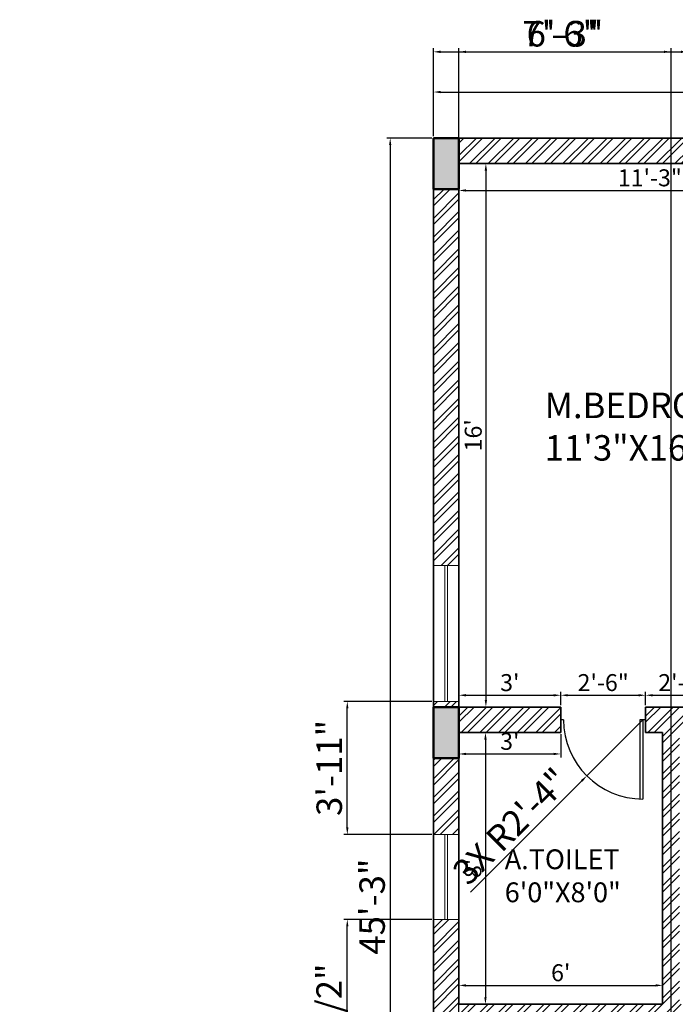
# Model space of a CAD drawing. Units: inches. Extents: x 4153 to 5577, y 785 to 1503.
# Tile 8 of 11: x 4865 to 5097, y 1138 to 1486. Entities that reach past the tile are written whole.
import ezdxf

# ---------------------------------------------------------------- set-up
doc = ezdxf.new("R2010")
doc.units = ezdxf.units.IN
for name, color, linetype, lineweight in [('A-ANNO-DIMS', 2, 'Continuous', 18), ('A-AREA-IDEN', 7, 'Continuous', 25), ('A-COLS', 7, 'Continuous', 50), ('A-DOOR', 3, 'Continuous', 25), ('A-GLAZ', 4, 'Continuous', 18), ('A-WALL', 7, 'Continuous', 35)]:
    doc.layers.add(name, color=color, linetype=linetype, lineweight=lineweight)
doc.layers.add('A-WALL-PATT', color=251, linetype='Continuous', lineweight=13, true_color=0x636466)
doc.styles.get("Standard").update_dxf_attribs({"font": 'arial.ttf'})
doc.dimstyles.new('ISO-25', dxfattribs={"dimtxt": 9, "dimasz": 2.5, "dimexe": 1.25, "dimexo": 0.625, "dimtad": 1, "dimlunit": 3, "dimtxsty": 'Standard', "dimcen": 2.5, "dimadec": 0, "dimazin": 0, "dimtfac": 1, "dimtmove": 0, "dimatfit": 3, "dimfxl": 1, "dimarcsym": 0})

# ---------------------------------------------------------------- blocks, each defined once
blk = doc.blocks.new('D2')
for p, q in [((1, 0), (1, 28)), ((2, 0), (2, 27.98)), ((0, 0), (2, 0)), ((29, 0), (30, 0))]:
    blk.add_line(p, q)
at = {"ltscale": 0.5}
blk.add_arc((1, 0), 28, 0, 90, dxfattribs=at)
blk = doc.blocks.new('*D23')
at = {"layer": 'A-ANNO-DIMS', "color": 0, "lineweight": -2, "transparency": 16777216}
for p, q in [((5011.25, 1445.11), (5011.25, 1461.99)), ((5518.25, 1445.11), (5518.25, 1461.99)), ((5013.75, 1460.74), (5515.75, 1460.74))]:
    blk.add_line(p, q, dxfattribs=at)
at = {"layer": 'A-ANNO-DIMS', "color": 0, "transparency": 16777216}
for points in [[(5013.75, 1461.16), (5013.75, 1460.33), (5011.25, 1460.74)], [(5515.75, 1461.16), (5515.75, 1460.33), (5518.25, 1460.74)]]:
    blk.add_solid(points, dxfattribs=at)
at = {"layer": 'Defpoints', "color": 0, "transparency": 16777216}
for p in [(5518.25, 1460.74), (5011.25, 1444.49), (5518.25, 1444.49)]:
    blk.add_point(p, dxfattribs=at)
at = {"layer": 'A-ANNO-DIMS', "color": 0, "transparency": 16777216, "insert": (5264.75, 1465.97), "char_height": 9, "attachment_point": 5}
blk.add_mtext('42\'-3"', dxfattribs=at)
blk = doc.blocks.new('*D24')
at = {"layer": 'A-ANNO-DIMS', "color": 0, "lineweight": -2, "transparency": 16777216}
for p, q in [((5010.63, 1444.49), (4994.72, 1444.49)), ((4995.97, 1441.99), (4995.97, 903.99)), ((5010.63, 901.49), (4994.72, 901.49))]:
    blk.add_line(p, q, dxfattribs=at)
at = {"layer": 'A-ANNO-DIMS', "color": 0, "transparency": 16777216}
for points in [[(4995.55, 1441.99), (4996.38, 1441.99), (4995.97, 1444.49)], [(4995.55, 903.99), (4996.38, 903.99), (4995.97, 901.49)]]:
    blk.add_solid(points, dxfattribs=at)
at = {"layer": 'Defpoints', "color": 0, "transparency": 16777216}
for p in [(5011.25, 1444.49), (4995.97, 901.49), (5011.25, 901.49)]:
    blk.add_point(p, dxfattribs=at)
at = {"layer": 'A-ANNO-DIMS', "color": 0, "transparency": 16777216, "insert": (4990.74, 1172.99), "char_height": 9, "attachment_point": 5, "rotation": 90}
blk.add_mtext('45\'-3"', dxfattribs=at)
blk = doc.blocks.new('*D25')
at = {"layer": 'A-ANNO-DIMS', "color": 0, "lineweight": -2, "transparency": 16777216}
for p, q in [((5020.25, 1434.86), (5020.25, 1424.72)), ((5155.25, 1434.86), (5155.25, 1424.72)), ((5022.75, 1425.97), (5152.75, 1425.97))]:
    blk.add_line(p, q, dxfattribs=at)
at = {"layer": 'A-ANNO-DIMS', "color": 0, "transparency": 16777216}
for points in [[(5022.75, 1426.39), (5022.75, 1425.56), (5020.25, 1425.97)], [(5152.75, 1426.39), (5152.75, 1425.56), (5155.25, 1425.97)]]:
    blk.add_solid(points, dxfattribs=at)
at = {"layer": 'Defpoints', "color": 0, "transparency": 16777216}
for p in [(5020.25, 1435.49), (5155.25, 1435.49), (5155.25, 1425.97)]:
    blk.add_point(p, dxfattribs=at)
at = {"layer": 'A-ANNO-DIMS', "color": 0, "transparency": 16777216, "insert": (5087.75, 1429.66), "char_height": 6, "attachment_point": 5}
blk.add_mtext('11\'-3"', dxfattribs=at)
blk = doc.blocks.new('*D26')
at = {"layer": 'A-ANNO-DIMS', "color": 0, "lineweight": -2, "transparency": 16777216}
for p, q in [((5020.88, 1435.49), (5031.04, 1435.49)), ((5029.79, 1432.99), (5029.79, 1245.99)), ((5020.88, 1243.49), (5031.04, 1243.49))]:
    blk.add_line(p, q, dxfattribs=at)
at = {"layer": 'A-ANNO-DIMS', "color": 0, "transparency": 16777216}
for points in [[(5029.37, 1432.99), (5030.21, 1432.99), (5029.79, 1435.49)], [(5029.37, 1245.99), (5030.21, 1245.99), (5029.79, 1243.49)]]:
    blk.add_solid(points, dxfattribs=at)
at = {"layer": 'Defpoints', "color": 0, "transparency": 16777216}
for p in [(5020.25, 1435.49), (5020.25, 1243.49), (5029.79, 1243.49)]:
    blk.add_point(p, dxfattribs=at)
at = {"layer": 'A-ANNO-DIMS', "color": 0, "transparency": 16777216, "insert": (5026.1, 1339.49), "char_height": 6, "attachment_point": 5, "rotation": 90}
blk.add_mtext("16'", dxfattribs=at)
blk = doc.blocks.new('*D27')
at = {"layer": 'A-ANNO-DIMS', "color": 0, "lineweight": -2, "transparency": 16777216}
for p, q in [((5020.25, 1244.11), (5020.25, 1248.91)), ((5056.25, 1244.11), (5056.25, 1248.91)), ((5022.75, 1247.66), (5053.75, 1247.66))]:
    blk.add_line(p, q, dxfattribs=at)
at = {"layer": 'A-ANNO-DIMS', "color": 0, "transparency": 16777216}
for points in [[(5022.75, 1248.07), (5022.75, 1247.24), (5020.25, 1247.66)], [(5053.75, 1248.07), (5053.75, 1247.24), (5056.25, 1247.66)]]:
    blk.add_solid(points, dxfattribs=at)
at = {"layer": 'Defpoints', "color": 0, "transparency": 16777216}
for p in [(5056.25, 1247.66), (5020.25, 1243.49), (5056.25, 1243.49)]:
    blk.add_point(p, dxfattribs=at)
at = {"layer": 'A-ANNO-DIMS', "color": 0, "transparency": 16777216, "insert": (5038.25, 1251.35), "char_height": 6, "attachment_point": 5}
blk.add_mtext("3'", dxfattribs=at)
blk = doc.blocks.new('*D28')
at = {"layer": 'A-ANNO-DIMS', "color": 0, "lineweight": -2, "transparency": 16777216}
for p, q in [((5056.25, 1244.11), (5056.25, 1248.91)), ((5086.25, 1244.11), (5086.25, 1248.91)), ((5058.75, 1247.66), (5083.75, 1247.66))]:
    blk.add_line(p, q, dxfattribs=at)
at = {"layer": 'A-ANNO-DIMS', "color": 0, "transparency": 16777216}
for points in [[(5058.75, 1248.07), (5058.75, 1247.24), (5056.25, 1247.66)], [(5083.75, 1248.07), (5083.75, 1247.24), (5086.25, 1247.66)]]:
    blk.add_solid(points, dxfattribs=at)
at = {"layer": 'Defpoints', "color": 0, "transparency": 16777216}
for p in [(5086.25, 1247.66), (5056.25, 1243.49), (5086.25, 1243.49)]:
    blk.add_point(p, dxfattribs=at)
at = {"layer": 'A-ANNO-DIMS', "color": 0, "transparency": 16777216, "insert": (5071.25, 1251.35), "char_height": 6, "attachment_point": 5}
blk.add_mtext('2\'-6"', dxfattribs=at)
blk = doc.blocks.new('*D29')
at = {"layer": 'A-ANNO-DIMS', "color": 0, "lineweight": -2, "transparency": 16777216}
for p, q in [((5086.25, 1244.11), (5086.25, 1248.91)), ((5113.25, 1244.11), (5113.25, 1248.91)), ((5088.75, 1247.66), (5110.75, 1247.66))]:
    blk.add_line(p, q, dxfattribs=at)
at = {"layer": 'A-ANNO-DIMS', "color": 0, "transparency": 16777216}
for points in [[(5088.75, 1248.07), (5088.75, 1247.24), (5086.25, 1247.66)], [(5110.75, 1248.07), (5110.75, 1247.24), (5113.25, 1247.66)]]:
    blk.add_solid(points, dxfattribs=at)
at = {"layer": 'Defpoints', "color": 0, "transparency": 16777216}
for p in [(5113.25, 1247.66), (5086.25, 1243.49), (5113.25, 1243.49)]:
    blk.add_point(p, dxfattribs=at)
at = {"layer": 'A-ANNO-DIMS', "color": 0, "transparency": 16777216, "insert": (5099.75, 1251.35), "char_height": 6, "attachment_point": 5}
blk.add_mtext('2\'-3"', dxfattribs=at)
blk = doc.blocks.new('*D41')
at = {"layer": 'A-ANNO-DIMS', "color": 0, "lineweight": -2, "transparency": 16777216}
for p, q in [((5020.25, 1233.86), (5020.25, 1225.67)), ((5056.25, 1233.86), (5056.25, 1225.67)), ((5022.75, 1226.92), (5053.75, 1226.92))]:
    blk.add_line(p, q, dxfattribs=at)
at = {"layer": 'A-ANNO-DIMS', "color": 0, "transparency": 16777216}
for points in [[(5022.75, 1227.34), (5022.75, 1226.51), (5020.25, 1226.92)], [(5053.75, 1227.34), (5053.75, 1226.51), (5056.25, 1226.92)]]:
    blk.add_solid(points, dxfattribs=at)
at = {"layer": 'Defpoints', "color": 0, "transparency": 16777216}
for p in [(5020.25, 1234.49), (5056.25, 1234.49), (5056.25, 1226.92)]:
    blk.add_point(p, dxfattribs=at)
at = {"layer": 'A-ANNO-DIMS', "color": 0, "transparency": 16777216, "insert": (5038.25, 1230.61), "char_height": 6, "attachment_point": 5}
blk.add_mtext("3'", dxfattribs=at)
blk = doc.blocks.new('*D42')
at = {"layer": 'A-ANNO-DIMS', "color": 0, "lineweight": -2, "transparency": 16777216}
for p, q in [((5020.88, 1234.49), (5030.89, 1234.49)), ((5029.64, 1231.99), (5029.64, 1140.99)), ((5020.88, 1138.49), (5030.89, 1138.49))]:
    blk.add_line(p, q, dxfattribs=at)
at = {"layer": 'A-ANNO-DIMS', "color": 0, "transparency": 16777216}
for points in [[(5029.22, 1231.99), (5030.06, 1231.99), (5029.64, 1234.49)], [(5029.22, 1140.99), (5030.06, 1140.99), (5029.64, 1138.49)]]:
    blk.add_solid(points, dxfattribs=at)
at = {"layer": 'Defpoints', "color": 0, "transparency": 16777216}
for p in [(5020.25, 1234.49), (5020.25, 1138.49), (5029.64, 1138.49)]:
    blk.add_point(p, dxfattribs=at)
at = {"layer": 'A-ANNO-DIMS', "color": 0, "transparency": 16777216, "insert": (5025.95, 1186.49), "char_height": 6, "attachment_point": 5, "rotation": 90}
blk.add_mtext("8'", dxfattribs=at)
blk = doc.blocks.new('*D43')
at = {"layer": 'A-ANNO-DIMS', "color": 0, "lineweight": -2, "transparency": 16777216}
for p, q in [((5020.25, 1139.11), (5020.25, 1146.42)), ((5022.75, 1145.17), (5089.75, 1145.17)), ((5092.25, 1139.11), (5092.25, 1146.42))]:
    blk.add_line(p, q, dxfattribs=at)
at = {"layer": 'A-ANNO-DIMS', "color": 0, "transparency": 16777216}
for points in [[(5022.75, 1145.59), (5022.75, 1144.75), (5020.25, 1145.17)], [(5089.75, 1145.59), (5089.75, 1144.75), (5092.25, 1145.17)]]:
    blk.add_solid(points, dxfattribs=at)
at = {"layer": 'Defpoints', "color": 0, "transparency": 16777216}
for p in [(5092.25, 1145.17), (5020.25, 1138.49), (5092.25, 1138.49)]:
    blk.add_point(p, dxfattribs=at)
at = {"layer": 'A-ANNO-DIMS', "color": 0, "transparency": 16777216, "insert": (5056.25, 1148.86), "char_height": 6, "attachment_point": 5}
blk.add_mtext("6'", dxfattribs=at)
blk = doc.blocks.new('WINDOW-48IN')
for p, q in [((0, 9), (0, 0)), ((48, 9), (48, 0)), ((0, 5), (48, 5)), ((0, 4), (48, 4))]:
    blk.add_line(p, q)
blk = doc.blocks.new('VENT-WINDOW-30IN')
for p, q in [((9, 30), (0, 30)), ((4, 0), (4, 30)), ((5, 0), (5, 30)), ((9, 0), (0, 0))]:
    blk.add_line(p, q)
blk = doc.blocks.new('COL-9X18IN')
at = {"transparency": 33554687}
h = blk.add_hatch(color=256, dxfattribs=at)
h.dxf.hatch_style = 1
h.paths.add_polyline_path([(9, 18), (0, 18), (0, 0), (9, 0)])
blk.add_lwpolyline([(0, 18), (9, 18), (9, 0), (0, 0)], close=True)
blk = doc.blocks.new('*D146')
at = {"layer": 'A-ANNO-DIMS', "color": 0, "lineweight": -2, "transparency": 16777216}
for p, q in [((5011.25, 1445.11), (5011.25, 1476.19)), ((5013.75, 1474.94), (5098.75, 1474.94)), ((5101.25, 1445.11), (5101.25, 1476.19))]:
    blk.add_line(p, q, dxfattribs=at)
at = {"layer": 'A-ANNO-DIMS', "color": 0, "transparency": 16777216}
for points in [[(5013.75, 1475.36), (5013.75, 1474.52), (5011.25, 1474.94)], [(5098.75, 1475.36), (5098.75, 1474.52), (5101.25, 1474.94)]]:
    blk.add_solid(points, dxfattribs=at)
at = {"layer": 'Defpoints', "color": 0, "transparency": 16777216}
for p in [(5101.25, 1474.94), (5011.25, 1444.49), (5101.25, 1444.49)]:
    blk.add_point(p, dxfattribs=at)
at = {"layer": 'A-ANNO-DIMS', "color": 0, "transparency": 16777216, "insert": (5056.25, 1480.16), "char_height": 9, "attachment_point": 5}
blk.add_mtext('7\'-6"', dxfattribs=at)
blk = doc.blocks.new('*D151')
at = {"layer": 'A-ANNO-DIMS', "color": 0, "lineweight": -2, "transparency": 16777216}
for p, q in [((5010.63, 1168.49), (4979.55, 1168.49)), ((4980.8, 1091.49), (4980.8, 1165.99)), ((5010.63, 1088.99), (4979.55, 1088.99))]:
    blk.add_line(p, q, dxfattribs=at)
at = {"layer": 'A-ANNO-DIMS', "color": 0, "transparency": 16777216}
for points in [[(4980.39, 1165.99), (4981.22, 1165.99), (4980.8, 1168.49)], [(4980.39, 1091.49), (4981.22, 1091.49), (4980.8, 1088.99)]]:
    blk.add_solid(points, dxfattribs=at)
at = {"layer": 'Defpoints', "color": 0, "transparency": 16777216}
for p in [(4980.8, 1168.49), (5011.25, 1168.49), (5011.25, 1088.99)]:
    blk.add_point(p, dxfattribs=at)
at = {"layer": 'A-ANNO-DIMS', "color": 0, "transparency": 16777216, "insert": (4975.53, 1128.74), "char_height": 9, "attachment_point": 5, "rotation": 90}
blk.add_mtext('6\'-7 1/2"', dxfattribs=at)
blk = doc.blocks.new('*D152')
at = {"layer": 'A-ANNO-DIMS', "color": 0, "lineweight": -2, "transparency": 16777216}
for p, q in [((5010.63, 1245.49), (4979.55, 1245.49)), ((4980.8, 1200.99), (4980.8, 1242.99)), ((5010.63, 1198.49), (4979.55, 1198.49))]:
    blk.add_line(p, q, dxfattribs=at)
at = {"layer": 'A-ANNO-DIMS', "color": 0, "transparency": 16777216}
for points in [[(4980.39, 1242.99), (4981.22, 1242.99), (4980.8, 1245.49)], [(4980.39, 1200.99), (4981.22, 1200.99), (4980.8, 1198.49)]]:
    blk.add_solid(points, dxfattribs=at)
at = {"layer": 'Defpoints', "color": 0, "transparency": 16777216}
for p in [(4980.8, 1245.49), (5011.25, 1245.49), (5011.25, 1198.49)]:
    blk.add_point(p, dxfattribs=at)
at = {"layer": 'A-ANNO-DIMS', "color": 0, "transparency": 16777216, "insert": (4975.58, 1221.99), "char_height": 9, "attachment_point": 5, "rotation": 90}
blk.add_mtext('3\'-11"', dxfattribs=at)
blk = doc.blocks.new('*D156')
at = {"layer": 'A-ANNO-DIMS', "color": 0, "lineweight": -2, "transparency": 16777216}
for p, q in [((5020.25, 1001.11), (5020.25, 1476.19)), ((5022.75, 1474.94), (5092.75, 1474.94)), ((5095.25, 1001.11), (5095.25, 1476.19))]:
    blk.add_line(p, q, dxfattribs=at)
at = {"layer": 'A-ANNO-DIMS', "color": 0, "transparency": 16777216}
for points in [[(5022.75, 1475.36), (5022.75, 1474.52), (5020.25, 1474.94)], [(5092.75, 1475.36), (5092.75, 1474.52), (5095.25, 1474.94)]]:
    blk.add_solid(points, dxfattribs=at)
at = {"layer": 'Defpoints', "color": 0, "transparency": 16777216}
for p in [(5095.25, 1474.94), (5020.25, 1000.49), (5095.25, 1000.49)]:
    blk.add_point(p, dxfattribs=at)
at = {"layer": 'A-ANNO-DIMS', "color": 0, "transparency": 16777216, "insert": (5057.75, 1480.16), "char_height": 9, "attachment_point": 5}
blk.add_mtext('6\'-3"', dxfattribs=at)
blk = doc.blocks.new('*D162')
at = {"layer": 'A-ANNO-DIMS', "color": 0, "lineweight": -2, "transparency": 16777216}
for p, q in [((5085.25, 1238.99), (5065.46, 1219.19)), ((5024.36, 1178.09), (5063.69, 1217.42))]:
    blk.add_line(p, q, dxfattribs=at)
at = {"layer": 'A-ANNO-DIMS', "color": 0, "transparency": 16777216}
blk.add_solid([(5063.39, 1217.72), (5063.98, 1217.13), (5065.46, 1219.19)], dxfattribs=at)
at = {"layer": 'Defpoints', "color": 0, "transparency": 16777216}
for p in [(5085.25, 1238.99), (5065.46, 1219.19)]:
    blk.add_point(p, dxfattribs=at)
at = {"layer": 'A-ANNO-DIMS', "color": 0, "transparency": 16777216, "insert": (5039.45, 1200.57), "char_height": 9, "attachment_point": 5, "rotation": 45.0008}
blk.add_mtext('3X R2\'-4"', dxfattribs=at)

msp = doc.modelspace()

# ---------------------------------------------------------------- hatches: boundary and pattern name
at = {"layer": 'A-WALL-PATT', "transparency": 33554687}
h = msp.add_hatch(dxfattribs=at)
h.set_pattern_fill('ANSI32', color=256, scale=0.49)
h.set_pattern_definition([(45, (816.3263, 0), (-3.300244, 3.300244), []), (45, (818.5265, 0), (-3.300244, 3.300244), [])])
h.paths.add_polyline_path([(5011.254, 1088.988), (5020.254, 1088.988), (5020.254, 1129.488), (5155.254, 1129.488), (5155.254, 1105.488), (5161.254, 1105.488), (5161.254, 1138.488), (5098.254, 1138.488), (5098.254, 1234.488), (5113.254, 1234.488), (5113.254, 1243.488), (5086.254, 1243.488), (5086.254, 1234.488), (5092.254, 1234.488), (5092.254, 1138.488), (5020.254, 1138.488), (5020.254, 1168.488), (5011.254, 1168.488)])
h.paths.add_polyline_path([(5011.254, 1009.488), (5020.254, 1009.488), (5020.254, 1040.988), (5011.254, 1040.988)])
h.paths.add_polyline_path([(5095.254, 991.488), (5095.254, 1000.488), (5020.254, 1000.488), (5020.254, 991.488)])
h.paths.add_polyline_path([(5011.254, 910.488), (5020.254, 910.488), (5020.254, 991.488), (5011.254, 991.488)])
h.paths.add_polyline_path([(5152.254, 901.488), (5152.254, 907.488), (5020.254, 907.488), (5020.254, 901.488)])
h.paths.add_polyline_path([(5161.254, 1057.488), (5155.254, 1057.488), (5155.254, 1000.488), (5161.254, 1000.488)])
h.paths.add_polyline_path([(5143.254, 991.488), (5152.254, 991.488), (5152.254, 1000.488), (5143.254, 1000.488)])
h.paths.add_polyline_path([(5161.254, 1000.488), (5161.254, 991.488), (5185.254, 991.488), (5185.254, 1000.488)])
h.paths.add_polyline_path([(5257.254, 991.488), (5257.254, 1000.488), (5233.254, 1000.488), (5233.254, 991.488)])
h.paths.add_polyline_path([(5266.254, 1120.488), (5257.254, 1120.488), (5257.254, 1000.488), (5266.254, 1000.488)])
h.paths.add_polyline_path([(5290.254, 991.488), (5290.254, 1000.488), (5275.254, 1000.488), (5275.254, 991.488)])
h.paths.add_polyline_path([(5362.254, 1000.488), (5362.254, 991.488), (5455.254, 991.488), (5455.254, 1000.488)])
h.paths.add_polyline_path([(5509.254, 1009.488), (5518.254, 1009.488), (5518.254, 1036.488), (5509.254, 1036.488)])
h.paths.add_polyline_path([(5503.254, 1000.488), (5503.254, 991.488), (5509.254, 991.488), (5509.254, 1000.488)])
h.paths.add_polyline_path([(5518.254, 1132.488), (5509.254, 1132.488), (5509.254, 1108.488), (5518.254, 1108.488)])
h.paths.add_polyline_path([(5509.254, 1204.488), (5518.254, 1204.488), (5518.254, 1225.488), (5509.254, 1225.488)])
h.paths.add_polyline_path([(5467.254, 1234.488), (5467.254, 1243.488), (5377.254, 1243.488), (5377.254, 1265.228), (5377.254, 1381.488), (5467.254, 1381.488), (5467.254, 1393.488), (5461.254, 1393.488), (5461.254, 1387.488), (5377.254, 1387.488), (5377.254, 1435.488), (5368.254, 1435.488), (5368.254, 1354.488), (5347.254, 1354.488), (5347.254, 1348.488), (5368.254, 1348.488), (5368.254, 1309.488), (5302.254, 1309.488), (5302.254, 1234.488), (5321.754, 1234.488), (5321.754, 1243.488), (5311.254, 1243.488), (5311.254, 1303.488), (5368.254, 1303.488), (5368.254, 1243.488), (5357.754, 1243.488), (5357.754, 1234.488)])
h.paths.add_polyline_path([(5509.254, 1357.488), (5518.254, 1357.488), (5518.254, 1426.488), (5509.254, 1426.488)])
h.paths.add_polyline_path([(5509.254, 1243.488), (5518.254, 1243.488), (5518.254, 1309.488), (5509.254, 1309.488)])
h.paths.add_polyline_path([(5509.254, 1435.488), (5509.254, 1444.488), (5425.254, 1444.488), (5425.254, 1435.488), (5461.254, 1435.488), (5461.254, 1423.488), (5467.254, 1423.488), (5467.254, 1435.488)])
h.paths.add_polyline_path([(5302.254, 1435.488), (5302.254, 1348.488), (5317.254, 1348.488), (5317.254, 1354.488), (5311.254, 1354.488), (5311.254, 1435.488), (5314.254, 1435.488), (5314.254, 1444.488), (5296.254, 1444.488), (5296.254, 1435.488)])
h.paths.add_polyline_path([(5368.254, 1444.488), (5362.254, 1444.488), (5362.254, 1435.488), (5368.254, 1435.488)])
h.paths.add_polyline_path([(5389.254, 1444.488), (5386.254, 1444.488), (5386.254, 1435.488), (5389.254, 1435.488)])
h.paths.add_polyline_path([(5248.254, 1435.488), (5248.254, 1444.488), (5173.254, 1444.488), (5173.254, 1435.488)])
h.paths.add_polyline_path([(5101.254, 1435.488), (5101.254, 1444.488), (5020.254, 1444.488), (5020.254, 1435.488)])
h.paths.add_polyline_path([(5011.254, 1293.488), (5020.254, 1293.488), (5020.254, 1295.242), (5020.254, 1426.488), (5011.254, 1426.488)])
h.paths.add_polyline_path([(5155.254, 1243.488), (5149.254, 1243.488), (5149.254, 1234.488), (5248.254, 1234.488), (5248.254, 1243.488), (5164.254, 1243.488), (5164.254, 1435.488), (5155.254, 1435.488)])
h.paths.add_polyline_path([(5020.254, 1243.488), (5020.254, 1234.488), (5056.254, 1234.488), (5056.254, 1243.488)], flags=17)
h.paths.add_polyline_path([(5020.254, 1225.488), (5011.254, 1225.488), (5011.254, 1198.488), (5020.254, 1198.488)], flags=17)
h = msp.add_hatch(dxfattribs=at)
h.set_pattern_fill('ANSI32', color=256, scale=0.5)
h.paths.add_polyline_path([(5020.254, 1245.488), (5011.254, 1245.488), (5011.254, 1243.488), (5020.254, 1243.488)])
h.paths.add_polyline_path([(4203.927, 1245.488), (4194.927, 1245.488), (4194.927, 1243.488), (4203.927, 1243.488)])

# ---------------------------------------------------------------- linework, layer by layer
at = {"layer": 'A-WALL'}
for p, q in [((5011.254, 1444.488), (5518.254, 1444.488)), ((5011.254, 901.488), (5011.254, 1444.488)), ((5020.254, 1435.488), (5155.254, 1435.488)), ((5020.254, 1243.488), (5020.254, 1435.488)), ((5020.254, 1243.488), (5056.254, 1243.488)), ((5056.254, 1234.488), (5056.254, 1243.488)), ((5086.254, 1243.488), (5113.254, 1243.488)), ((5086.254, 1234.488), (5086.254, 1243.488)), ((5020.254, 1234.488), (5056.254, 1234.488)), ((5020.254, 1138.488), (5020.254, 1234.488)), ((5086.254, 1234.488), (5092.254, 1234.488)), ((5092.254, 1138.488), (5092.254, 1234.488)), ((5020.254, 1138.488), (5092.254, 1138.488))]:
    msp.add_line(p, q, dxfattribs=at)

# ---------------------------------------------------------------- block references
at = {"layer": 'A-COLS'}
for p in [(5011.254, 1426.488), (5011.254, 1225.488)]:
    msp.add_blockref('COL-9X18IN', p, dxfattribs=at)
at = {"layer": 'A-DOOR', "rotation": 180}
msp.add_blockref('D2', (5086.254, 1238.988), dxfattribs=at)
at = {"layer": 'A-GLAZ', "rotation": 269.9999999999995}
msp.add_blockref('WINDOW-48IN', (5011.254, 1293.488), dxfattribs=at)
at = {"layer": 'A-GLAZ'}
msp.add_blockref('VENT-WINDOW-30IN', (5011.254, 1168.488), dxfattribs=at)

# ---------------------------------------------------------------- texts
at = {"layer": 'A-AREA-IDEN', "attachment_point": 1}
for s, insert, char_height in [('{\\fTimes New Roman|b0|i0|c0|p18;M.BEDROOM\\P11\'3"X16\'0"}', (5050.587, 1354.548), 9), ('{\\fTimes New Roman|b0|i0|c0|p18;A.TOILET\\P6\'0"X8\'0"}', (5036.462, 1193.216), 7)]:
    msp.add_mtext_dynamic_manual_height_columns(s, width=67.35079, gutter_width=12.5, heights=[0], dxfattribs=dict(at, insert=insert, char_height=char_height))

# ---------------------------------------------------------------- dimensions: what is measured, and where the dimension line sits
at = {"layer": 'A-ANNO-DIMS'}
for base, p1, p2, override, picture, middle in [((5101.254, 1474.938), (5011.254, 1444.488), (5101.254, 1444.488), {"dimdec": 1, "dimlfac": 1, "dimrnd": 0, "dimzin": 1, "dimdsep": 46, "dimlunit": 4, "dimfrac": 2}, '*D146', (5056.254, 1480.159)), ((5095.254, 1474.938), (5020.254, 1000.488), (5095.254, 1000.488), {"dimdec": 1, "dimlfac": 1, "dimrnd": 0, "dimzin": 1, "dimdsep": 46, "dimlunit": 4, "dimfrac": 2}, '*D156', (5057.754, 1480.162)), ((5518.254, 1460.744), (5011.254, 1444.488), (5518.254, 1444.488), {"dimclrd": 0, "dimclre": 0, "dimclrt": 0}, '*D23', (5264.754, 1465.968)), ((5155.254, 1425.974), (5020.254, 1435.488), (5155.254, 1435.488), {"dimtxt": 6, "dimclrd": 0, "dimclre": 0, "dimclrt": 0}, '*D25', (5087.754, 1429.665)), ((5056.254, 1247.658), (5020.254, 1243.488), (5056.254, 1243.488), {"dimtxt": 6, "dimclrd": 0, "dimclre": 0, "dimclrt": 0}, '*D27', (5038.254, 1251.349)), ((5086.254, 1247.658), (5056.254, 1243.488), (5086.254, 1243.488), {"dimtxt": 6, "dimclrd": 0, "dimclre": 0, "dimclrt": 0, "dimtmove": 1}, '*D28', (5071.254, 1251.347)), ((5113.254, 1247.658), (5086.254, 1243.488), (5113.254, 1243.488), {"dimtxt": 6, "dimclrd": 0, "dimclre": 0, "dimclrt": 0, "dimtmove": 1}, '*D29', (5099.754, 1251.349)), ((5056.254, 1226.923), (5020.254, 1234.488), (5056.254, 1234.488), {"dimtxt": 6, "dimclrd": 0, "dimclre": 0, "dimclrt": 0}, '*D41', (5038.254, 1230.614)), ((5092.254, 1145.169), (5020.254, 1138.488), (5092.254, 1138.488), {"dimtxt": 6, "dimclrd": 0, "dimclre": 0, "dimclrt": 0}, '*D43', (5056.254, 1148.858))]:
    dim = msp.add_linear_dim(base=base, p1=p1, p2=p2, dimstyle='ISO-25', override=override, dxfattribs=at)
    dim.commit()
    dim.dimension.update_dxf_attribs({"geometry": picture, "text_midpoint": middle})
for base, p1, p2, override, picture, middle in [((4995.968, 901.488), (5011.254, 1444.488), (5011.254, 901.488), {"dimclrd": 0, "dimclre": 0, "dimclrt": 0}, '*D24', (4990.745, 1172.988)), ((5029.791, 1243.488), (5020.254, 1435.488), (5020.254, 1243.488), {"dimtxt": 6, "dimclrd": 0, "dimclre": 0, "dimclrt": 0}, '*D26', (5026.102, 1339.488)), ((4980.804, 1245.488), (5011.254, 1198.488), (5011.254, 1245.488), {"dimdec": 1, "dimlfac": 1, "dimrnd": 0, "dimzin": 1, "dimdsep": 46, "dimlunit": 4, "dimfrac": 2}, '*D152', (4975.581, 1221.988)), ((5029.64, 1138.488), (5020.254, 1234.488), (5020.254, 1138.488), {"dimtxt": 6, "dimclrd": 0, "dimclre": 0, "dimclrt": 0}, '*D42', (5025.951, 1186.488)), ((4980.804, 1168.488), (5011.254, 1088.988), (5011.254, 1168.488), {"dimdec": 1, "dimlfac": 1, "dimrnd": 0, "dimzin": 1, "dimdsep": 46, "dimlunit": 4, "dimfrac": 2}, '*D151', (4975.525, 1128.738))]:
    dim = msp.add_linear_dim(base=base, p1=p1, p2=p2, angle=90, dimstyle='ISO-25', override=override, dxfattribs=at)
    dim.commit()
    dim.dimension.update_dxf_attribs({"geometry": picture, "text_midpoint": middle})
dim = msp.add_radius_dim(center=(5085.254, 1238.988), mpoint=(5065.455, 1219.189), text='3X <>', dimstyle='ISO-25', override={"dimdec": 1, "dimlfac": 1, "dimrnd": 0, "dimzin": 1, "dimdsep": 46, "dimlunit": 4, "dimfrac": 2}, dxfattribs=at)
dim.commit()
dim.dimension.update_dxf_attribs({"geometry": '*D162', "text_midpoint": (5039.446, 1200.566)})

doc.saveas('drawing.dxf')
